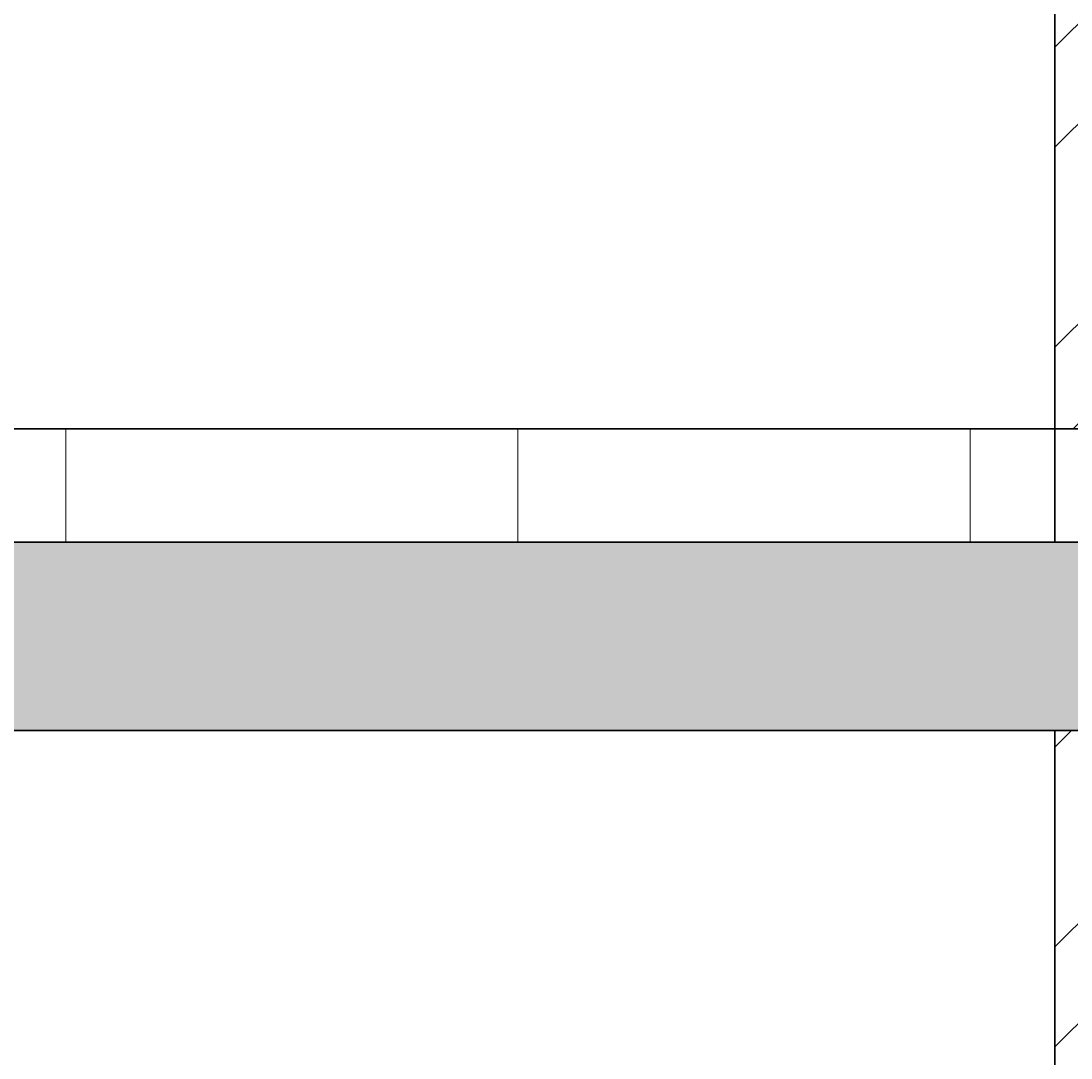
# Model space of a CAD drawing. Units: inches. Extents: x -301 to 715, y -607 to 364.
# Tile 47 of 141: x 107 to 135, y -370 to -343. Entities that reach past the tile are written whole.
import ezdxf

# ---------------------------------------------------------------- set-up
doc = ezdxf.new("R2010")
doc.units = ezdxf.units.IN
doc.header["$MEASUREMENT"] = 0
for name, color, linetype, lineweight in [('A-ANNO-DIMS', 2, 'Continuous', 18), ('A-SECT', 1, 'Continuous', 35), ('A-SECT-PATT', 8, 'Continuous', 13)]:
    doc.layers.add(name, color=color, linetype=linetype, lineweight=lineweight)
doc.styles.get("Standard").update_dxf_attribs({"font": 'arial.ttf'})
doc.dimstyles.get("Standard").update_dxf_attribs({"dimtxt": 0.18, "dimasz": 0.18, "dimexe": 0.18, "dimexo": 0.0625, "dimgap": 0.09, "dimtad": 0, "dimtih": 1, "dimtoh": 1, "dimdec": 1, "dimzin": 0, "dimdsep": 46, "dimlunit": 4, "dimtxsty": 'Standard', "dimcen": 0.09, "dimclrd": 3, "dimclre": 4, "dimclrt": 6, "dimadec": 0, "dimazin": 0, "dimtfac": 1, "dimtdec": 1, "dimtofl": 0, "dimtmove": 0, "dimatfit": 3, "dimfxl": 1, "dimtfill": 2, "dimtfillclr": 51, "dimtolj": 1, "dimtzin": 0, "dimarcsym": 0})

# ---------------------------------------------------------------- blocks, each defined once
blk = doc.blocks.new('*D176')
at = {"layer": 'A-ANNO-DIMS', "color": 4, "lineweight": -2, "transparency": 16777216}
for p, q in [((148.28, -324.477), (215.605, -324.477)), ((-15.22, -540.477), (215.605, -540.477))]:
    blk.add_line(p, q, dxfattribs=at)
at = {"layer": 'A-ANNO-DIMS', "color": 3, "lineweight": -2, "transparency": 16777216}
for p, q in [((215.425, -324.657), (215.425, -432.296)), ((215.425, -540.297), (215.425, -432.659))]:
    blk.add_line(p, q, dxfattribs=at)
at = {"layer": 'A-ANNO-DIMS', "color": 3, "transparency": 16777216}
for points in [[(215.395, -324.657), (215.455, -324.657), (215.425, -324.477)], [(215.395, -540.297), (215.455, -540.297), (215.425, -540.477)]]:
    blk.add_solid(points, dxfattribs=at)
at = {"layer": 'Defpoints', "color": 0, "transparency": 16777216}
for p in [(148.218, -324.477), (-15.282, -540.477), (215.425, -540.477)]:
    blk.add_point(p, dxfattribs=at)
at = {"layer": 'A-ANNO-DIMS', "color": 6, "transparency": 16777216, "insert": (215.425, -432.477), "char_height": 0.18, "attachment_point": 5, "bg_fill": 1, "box_fill_scale": 1.25, "bg_fill_color": 51, "bg_fill_transparency": 0}
blk.add_mtext('\\A1;18\'-0"', dxfattribs=at)
blk = doc.blocks.new('*D186')
at = {"layer": 'A-ANNO-DIMS', "color": 4, "lineweight": -2, "transparency": 16777216}
for p, q in [((134.255, -353.415), (134.255, -292.467)), ((143.218, -353.415), (143.218, -292.467))]:
    blk.add_line(p, q, dxfattribs=at)
at = {"layer": 'A-ANNO-DIMS', "color": 3, "lineweight": -2, "transparency": 16777216}
for p, q in [((134.435, -292.647), (138.407, -292.647)), ((143.038, -292.647), (139.066, -292.647))]:
    blk.add_line(p, q, dxfattribs=at)
at = {"layer": 'A-ANNO-DIMS', "color": 3, "transparency": 16777216}
for points in [[(134.435, -292.617), (134.435, -292.677), (134.255, -292.647)], [(143.038, -292.617), (143.038, -292.677), (143.218, -292.647)]]:
    blk.add_solid(points, dxfattribs=at)
at = {"layer": 'Defpoints', "color": 0, "transparency": 16777216}
for p in [(143.218, -292.647), (134.255, -353.477), (143.218, -353.477)]:
    blk.add_point(p, dxfattribs=at)
at = {"layer": 'A-ANNO-DIMS', "color": 6, "transparency": 16777216, "insert": (138.737, -292.647), "char_height": 0.18, "attachment_point": 5, "bg_fill": 1, "box_fill_scale": 1.25, "bg_fill_color": 51, "bg_fill_transparency": 0}
blk.add_mtext('\\A1;0\'-9"', dxfattribs=at)
blk = doc.blocks.new('*D189')
at = {"layer": 'A-ANNO-DIMS', "color": 4, "lineweight": -2, "transparency": 16777216}
for p, q in [((134.193, -353.477), (-266.112, -353.477)), ((134.193, -361.477), (-266.112, -361.477))]:
    blk.add_line(p, q, dxfattribs=at)
at = {"layer": 'A-ANNO-DIMS', "color": 3, "lineweight": -2, "transparency": 16777216}
for p, q in [((-265.932, -353.657), (-265.932, -357.296)), ((-265.932, -361.297), (-265.932, -357.659))]:
    blk.add_line(p, q, dxfattribs=at)
at = {"layer": 'A-ANNO-DIMS', "color": 3, "transparency": 16777216}
for points in [[(-265.962, -353.657), (-265.902, -353.657), (-265.932, -353.477)], [(-265.962, -361.297), (-265.902, -361.297), (-265.932, -361.477)]]:
    blk.add_solid(points, dxfattribs=at)
at = {"layer": 'Defpoints', "color": 0, "transparency": 16777216}
for p in [(134.255, -353.477), (-265.932, -361.477), (134.255, -361.477)]:
    blk.add_point(p, dxfattribs=at)
at = {"layer": 'A-ANNO-DIMS', "color": 6, "transparency": 16777216, "insert": (-265.932, -357.477), "char_height": 0.18, "attachment_point": 5, "bg_fill": 1, "box_fill_scale": 1.25, "bg_fill_color": 51, "bg_fill_transparency": 0}
blk.add_mtext('\\A1;0\'-8"', dxfattribs=at)

msp = doc.modelspace()

# ---------------------------------------------------------------- hatches: boundary and pattern name
at = {"layer": 'A-SECT-PATT'}
h = msp.add_hatch(dxfattribs=at)
h.set_pattern_fill('ANSI32', color=256, scale=15)
h.set_pattern_definition([(45, (10.321, 33.8764), (-3.977476, 3.977476), []), (45, (12.973, 33.8764), (-3.977476, 3.977476), [])])
h.paths.add_polyline_path([(-185.282, -324.477), (-199.282, -324.477), (-199.282, -329.477), (-194.282, -329.477), (-194.282, -353.477), (-185.282, -353.477)])
h.paths.add_polyline_path([(-185.282, -361.477), (-193.904, -361.477), (-193.982, -377.537), (-185.282, -377.537)])
h.paths.add_polyline_path([(143.218, -329.477), (148.218, -329.477), (148.218, -324.477), (134.255, -324.477), (134.255, -353.477), (143.218, -353.477)])
h.paths.add_polyline_path([(143.218, -361.477), (134.255, -361.477), (134.255, -377.477), (143.218, -377.477)])
h.paths.add_polyline_path([(-185.282, -439.477), (-194.282, -439.477), (-194.282, -463.477), (-185.282, -463.477)])
h.paths.add_polyline_path([(-185.282, -471.477), (-194.282, -471.477), (-194.282, -481.477), (-185.282, -481.477)])
h.paths.add_polyline_path([(-185.282, -463.477), (-194.282, -463.477), (-194.282, -466.477), (-185.282, -466.477)])
h.paths.add_polyline_path([(-185.282, -466.477), (-194.282, -466.477), (-194.282, -471.477), (-185.282, -471.477)])
h.paths.add_polyline_path([(-180.282, -481.477), (-185.282, -481.477), (-194.282, -481.477), (-199.282, -481.477), (-199.282, -493.477), (-180.282, -493.477)])
h.paths.add_polyline_path([(-175.282, -493.477), (-180.282, -493.477), (-199.282, -493.477), (-204.282, -493.477), (-204.282, -511.477), (-175.282, -511.477)])
h.paths.add_polyline_path([(-170.282, -511.477), (-175.282, -511.477), (-204.282, -511.477), (-209.282, -511.477), (-209.282, -535.477), (-170.282, -535.477)])
h.paths.add_polyline_path([(-35.282, -463.477), (-41.282, -463.477), (-41.282, -466.477), (-35.282, -466.477)])
h.paths.add_polyline_path([(-35.282, -466.477), (-41.282, -466.477), (-41.282, -471.477), (-35.282, -471.477)])
h.paths.add_polyline_path([(-35.282, -471.477), (-41.282, -471.477), (-41.282, -481.477), (-35.282, -481.477)])
h.paths.add_polyline_path([(-30.282, -481.477), (-46.282, -481.477), (-46.282, -493.477), (-30.282, -493.477)])
h.paths.add_polyline_path([(-25.282, -493.477), (-30.282, -493.477), (-46.282, -493.477), (-51.282, -493.477), (-51.282, -511.477), (-25.282, -511.477)])
h.paths.add_polyline_path([(-20.282, -511.477), (-25.282, -511.477), (-51.282, -511.477), (-56.282, -511.477), (-56.282, -535.477), (-20.282, -535.477)])
h.paths.add_polyline_path([(143.218, -463.477), (134.255, -463.477), (134.255, -466.477), (143.218, -466.477)])
h.paths.add_polyline_path([(143.218, -466.477), (134.255, -466.477), (134.255, -471.477), (143.218, -471.477)])
h.paths.add_polyline_path([(143.218, -471.477), (134.255, -471.477), (134.255, -481.477), (143.218, -481.477)])
h.paths.add_polyline_path([(148.255, -481.477), (143.255, -481.477), (134.255, -481.477), (129.255, -481.477), (129.255, -493.477), (148.255, -493.477)])
h.paths.add_polyline_path([(153.255, -493.477), (148.255, -493.477), (129.255, -493.477), (124.255, -493.477), (124.255, -511.477), (153.255, -511.477)])
h.paths.add_polyline_path([(158.255, -511.477), (153.255, -511.477), (124.255, -511.477), (119.255, -511.477), (119.255, -535.477), (158.255, -535.477)])
h = msp.add_hatch(dxfattribs=at)
h.set_pattern_fill('ANSI31', color=256, scale=96, angle=45, style=0)
h.paths.add_polyline_path([(-185.282, -356.477), (134.255, -356.477), (134.255, -353.477), (-185.282, -353.477)])
h = msp.add_hatch(dxfattribs=at)
h.set_pattern_fill('AR-CONC', color=256, scale=0.5)
h.set_pattern_definition([(50, (10.3213, 33.8764), (3.586301, -0.31376), [0.375, -4.125]), (355, (10.3213, 33.8764), (-0.693757, 3.76096), [0.3, -3.3]), (100.45144, (10.62, 33.8502), (2.892544, 3.4472), [0.3187, -3.50571]), (46.1842, (10.3213, 34.8764), (5.336207, -0.827596), [0.5625, -6.1875]), (96.6356, (10.766, 34.8074), (4.67331, 4.870593), [0.47805, -5.25857]), (351.1842, (10.321, 34.8764), (4.67331, 4.870593), [0.45, -4.95]), (21, (10.8213, 34.6264), (2.984535, -2.013094), [0.375, -4.125]), (326, (10.8213, 34.6264), (1.216577, 3.62575), [0.3, -3.3]), (71.45144, (11.07, 34.4586), (4.201112, 1.612656), [0.3187, -3.50571]), (37.5, (10.3213, 33.8764), (0.0607993, 1.6644693), [0, -3.26, 0, -3.35, 0, -3.3125]), (7.5, (10.3213, 33.8764), (1.3153477, 1.9720586), [0, -1.91, 0, -3.185, 0, -1.2625]), (327.5, (9.2063, 33.8764), (2.6691122, -0.1127744), [0, -1.25, 0, -3.9, 0, -5.175]), (317.5, (8.7063, 33.8764), (2.915931, 0.500525), [0, -1.625, 0, -2.59, 0, -3.675])])
h.paths.add_polyline_path([(-56.282, -535.477), (-61.282, -535.477), (-61.282, -540.477), (-15.282, -540.477), (-15.282, -535.477), (-20.282, -535.477)])
h.paths.add_polyline_path([(119.255, -535.477), (114.255, -535.477), (114.255, -540.477), (163.255, -540.477), (163.255, -535.477), (158.255, -535.477)])
h.paths.add_polyline_path([(-206.282, -471.477), (-209.282, -471.477), (-209.282, -481.477), (-206.282, -481.477), (-194.282, -481.477), (-194.282, -471.477)])
h.paths.add_polyline_path([(-41.282, -481.477), (-41.282, -471.477), (-185.282, -471.477), (-185.282, -481.477), (-180.282, -481.477)])
h.paths.add_polyline_path([(134.255, -481.477), (134.255, -471.477), (-35.282, -471.477), (-35.282, -481.477), (-30.282, -481.477)])
h.paths.add_polyline_path([(155.218, -481.477), (158.218, -481.477), (158.218, -471.477), (153.218, -471.477), (143.218, -471.477), (143.218, -481.477), (148.255, -481.477)])
h.paths.add_polyline_path([(-193.88, -356.477), (-193.904, -361.477), (143.218, -361.477), (143.218, -356.477)])

# ---------------------------------------------------------------- linework, layer by layer
at = {"layer": 'A-SECT'}
for p, q in [((134.255, -324.477), (134.255, -353.477)), ((-194.282, -353.477), (143.218, -353.477)), ((134.255, -353.477), (134.255, -356.477)), ((-194.282, -356.477), (143.218, -356.477)), ((-194.282, -361.477), (143.218, -361.477)), ((134.255, -361.477), (134.255, -481.477))]:
    msp.add_line(p, q, dxfattribs=at)

# ---------------------------------------------------------------- dimensions: what is measured, and where the dimension line sits
at = {"layer": 'A-ANNO-DIMS'}
dim = msp.add_linear_dim(base=(143.218, -292.647), p1=(134.255, -353.477), p2=(143.218, -353.477), dimstyle='Standard', override={"dimdec": 1, "dimlfac": 1, "dimrnd": 0, "dimzin": 1, "dimdsep": 46, "dimlunit": 4, "dimfrac": 2}, dxfattribs=at)
dim.commit()
dim.dimension.update_dxf_attribs({"geometry": '*D186', "text_midpoint": (138.737, -292.647)})
for base, p1, p2, picture, middle in [((215.425, -540.477), (148.218, -324.477), (-15.282, -540.477), '*D176', (215.425, -432.477)), ((-265.932, -361.477), (134.255, -353.477), (134.255, -361.477), '*D189', (-265.932, -357.477))]:
    dim = msp.add_linear_dim(base=base, p1=p1, p2=p2, angle=90, dimstyle='Standard', override={"dimdec": 1, "dimlfac": 1, "dimrnd": 0, "dimzin": 1, "dimdsep": 46, "dimlunit": 4, "dimfrac": 2}, dxfattribs=at)
    dim.commit()
    dim.dimension.update_dxf_attribs({"geometry": picture, "text_midpoint": middle})

doc.saveas('drawing.dxf')
